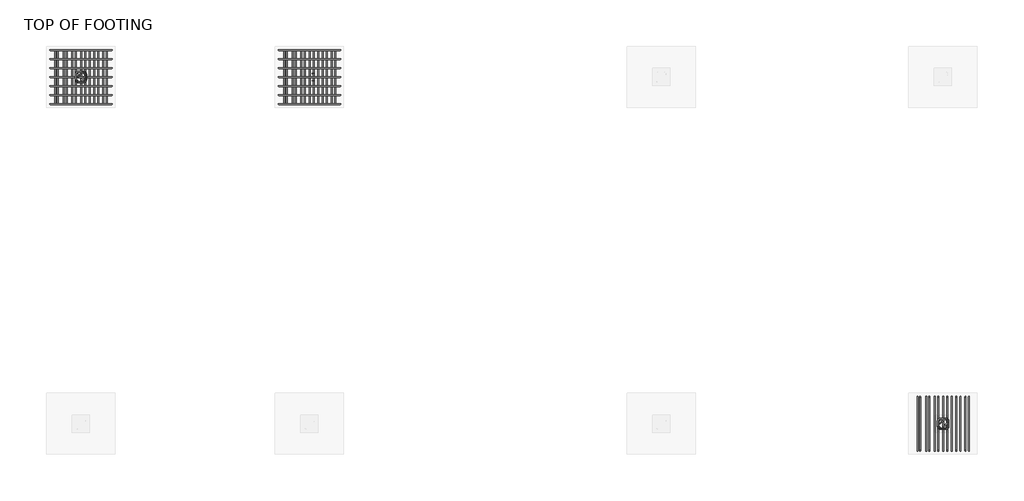
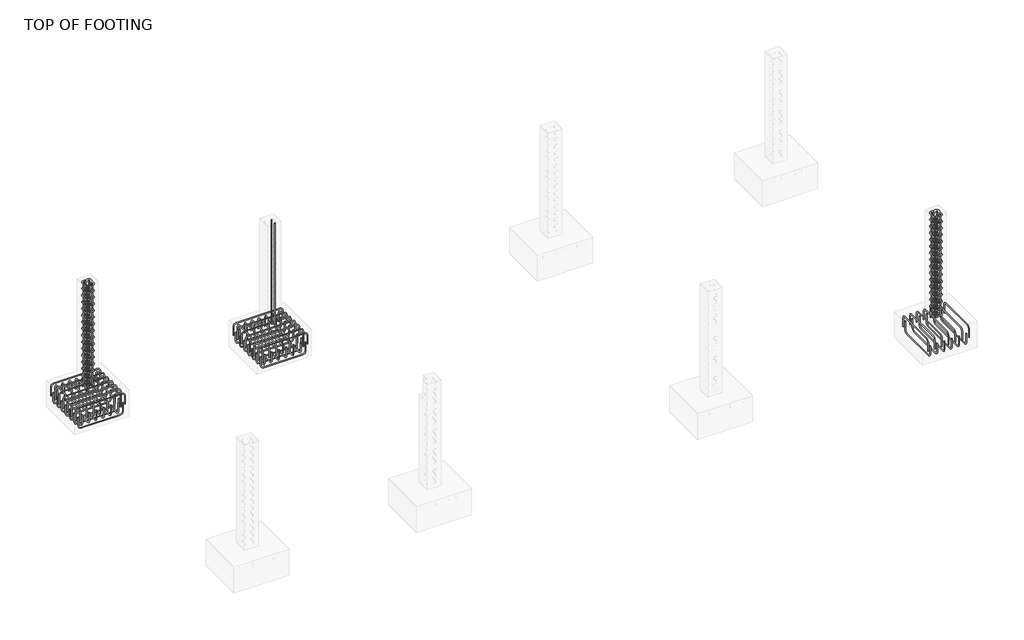
# One storey, part 5 of 6: 17 reinforcing bars.
"""IFC4 building model written with IfcOpenShell, lengths in millimetres."""

from ifc_helpers import new_model, si_unit, point, frame, origin, place, context, project, spatial, polyline, circle_curve, trimmed, segment, composite_curve, source, transform, mapped, element, save
from ifc_brep_helpers import swept_disk

model = new_model("IFC4")

# Units and contexts
model_context = context("Model", 3, world=origin())
ifc_project = project(units=[si_unit("LENGTHUNIT", "METRE", prefix="MILLI")], contexts=[model_context])

# Site, building, storey
site = spatial("IfcSite", under=ifc_project)
building = spatial("IfcBuilding", under=site)
storey = spatial("IfcBuildingStorey", under=building, Name="TOP OF FOOTING", Elevation=-1828.8)

# Reinforcing bars
placement = place(None, origin())
reinforcing_bar_shape = source(origin(), model_context, "Body", "SolidModel", [
    swept_disk(composite_curve([segment(polyline([(-14552.1855212, 4666.2516651, -2038.8), (-14552.1855212, 4666.2516651, -2186.1)]), True, "CONTINUOUS"), segment(trimmed(circle_curve(frame((-14598.5355212, 4666.2516651, -2186.1), z_axis=(0.0, 1.0, 0.0), x_axis=(46.350000000000364, 0.0, 0.0)), 46.35), [point((-14552.1855212, 4666.2516651, -2186.1))], [point((-14598.5355212, 4666.2516651, -2232.45))], True, "CARTESIAN"), True, "CONTINUOUS"), segment(polyline([(-14598.5355212, 4666.2516651, -2232.45), (-15241.6761323, 4666.2516651, -2232.45)]), True, "CONTINUOUS"), segment(trimmed(circle_curve(frame((-15241.6761323, 4666.2516651, -2186.1), z_axis=(0.0, 1.0, 0.0), x_axis=(0.0, 0.0, -46.34999999999991)), 46.35), [point((-15241.6761323, 4666.2516651, -2232.45))], [point((-15288.0261323, 4666.2516651, -2186.1))], True, "CARTESIAN"), True, "CONTINUOUS"), segment(polyline([(-15288.0261323, 4666.2516651, -2186.1), (-15288.0261323, 4666.2516651, -2038.8)]), True, "CONTINUOUS")], self_intersect=False), 6.35),
])
element("IfcReinforcingBar", 1, at=placement, inside=storey, context=model_context, shape_type="MappedRepresentation", body=[
    mapped(reinforcing_bar_shape, transform((0.0, 0.0, 0.0), x_axis=(1.0, 0.0, 0.0), y_axis=(0.0, 1.0, 0.0), z_axis=(0.0, 0.0, 1.0))),
    mapped(reinforcing_bar_shape, transform((0.0, -117.8833333, 0.0), x_axis=(1.0, 0.0, 0.0), y_axis=(0.0, 1.0, 0.0), z_axis=(0.0, 0.0, 1.0))),
    mapped(reinforcing_bar_shape, transform((0.0, -235.7666667, 0.0), x_axis=(1.0, 0.0, 0.0), y_axis=(0.0, 1.0, 0.0), z_axis=(0.0, 0.0, 1.0))),
    mapped(reinforcing_bar_shape, transform((0.0, -353.65, 0.0), x_axis=(1.0, 0.0, 0.0), y_axis=(0.0, 1.0, 0.0), z_axis=(0.0, 0.0, 1.0))),
    mapped(reinforcing_bar_shape, transform((0.0, -471.5333333, 0.0), x_axis=(1.0, 0.0, 0.0), y_axis=(0.0, 1.0, 0.0), z_axis=(0.0, 0.0, 1.0))),
    mapped(reinforcing_bar_shape, transform((0.0, -589.4166667, 0.0), x_axis=(1.0, 0.0, 0.0), y_axis=(0.0, 1.0, 0.0), z_axis=(0.0, 0.0, 1.0))),
    mapped(reinforcing_bar_shape, transform((0.0, -707.3, 0.0), x_axis=(1.0, 0.0, 0.0), y_axis=(0.0, 1.0, 0.0), z_axis=(0.0, 0.0, 1.0))),
])
reinforcing_bar_2_shape = source(origin(), model_context, "Body", "SolidModel", [
    swept_disk(composite_curve([segment(polyline([(-15327.4056799, 4666.2516651, -2070.9463075), (-15327.4056799, 4666.2516651, -1923.6463075)]), True, "CONTINUOUS"), segment(trimmed(circle_curve(frame((-15281.0556799, 4666.2516651, -1923.6463075), z_axis=(0.0, 1.0, 0.0), x_axis=(-46.350000000000364, 0.0, 0.0)), 46.35), [point((-15327.4056799, 4666.2516651, -1923.6463075))], [point((-15281.0556799, 4666.2516651, -1877.2963075))], True, "CARTESIAN"), True, "CONTINUOUS"), segment(polyline([(-15281.0556799, 4666.2516651, -1877.2963075), (-14566.4556799, 4666.2516651, -1877.2963075)]), True, "CONTINUOUS"), segment(trimmed(circle_curve(frame((-14566.4556799, 4666.2516651, -1923.6463075), z_axis=(0.0, 1.0, 0.0), x_axis=(0.0, 0.0, 46.34999999999991)), 46.35), [point((-14566.4556799, 4666.2516651, -1877.2963075))], [point((-14520.1056799, 4666.2516651, -1923.6463075))], True, "CARTESIAN"), True, "CONTINUOUS"), segment(polyline([(-14520.1056799, 4666.2516651, -1923.6463075), (-14520.1056799, 4666.2516651, -2070.9463075)]), True, "CONTINUOUS")], self_intersect=False), 6.35),
])
element("IfcReinforcingBar", 2, at=placement, inside=storey, context=model_context, shape_type="MappedRepresentation", body=[
    mapped(reinforcing_bar_2_shape, transform((0.0, 0.0, 0.0), x_axis=(1.0, 0.0, 0.0), y_axis=(0.0, 1.0, 0.0), z_axis=(0.0, 0.0, 1.0))),
    mapped(reinforcing_bar_2_shape, transform((0.0, -117.8833333, 0.0), x_axis=(1.0, 0.0, 0.0), y_axis=(0.0, 1.0, 0.0), z_axis=(0.0, 0.0, 1.0))),
    mapped(reinforcing_bar_2_shape, transform((0.0, -235.7666667, 0.0), x_axis=(1.0, 0.0, 0.0), y_axis=(0.0, 1.0, 0.0), z_axis=(0.0, 0.0, 1.0))),
    mapped(reinforcing_bar_2_shape, transform((0.0, -353.65, 0.0), x_axis=(1.0, 0.0, 0.0), y_axis=(0.0, 1.0, 0.0), z_axis=(0.0, 0.0, 1.0))),
    mapped(reinforcing_bar_2_shape, transform((0.0, -471.5333333, 0.0), x_axis=(1.0, 0.0, 0.0), y_axis=(0.0, 1.0, 0.0), z_axis=(0.0, 0.0, 1.0))),
    mapped(reinforcing_bar_2_shape, transform((0.0, -589.4166667, 0.0), x_axis=(1.0, 0.0, 0.0), y_axis=(0.0, 1.0, 0.0), z_axis=(0.0, 0.0, 1.0))),
    mapped(reinforcing_bar_2_shape, transform((0.0, -707.3, 0.0), x_axis=(1.0, 0.0, 0.0), y_axis=(0.0, 1.0, 0.0), z_axis=(0.0, 0.0, 1.0))),
])
reinforcing_bar_3_shape = source(origin(), model_context, "Body", "SolidModel", [
    swept_disk(composite_curve([segment(polyline([(-14585.2545962, 4666.2516651, -2094.0228735), (-14585.2545962, 4666.2516651, -1946.7228735)]), True, "CONTINUOUS"), segment(trimmed(circle_curve(frame((-14585.2545962, 4619.9016651, -1946.7228735), z_axis=(1.0, 0.0, 0.0), x_axis=(0.0, 46.349999999999454, 0.0)), 46.35), [point((-14585.2545962, 4666.2516651, -1946.7228735))], [point((-14585.2545962, 4619.9016651, -1900.3728735))], True, "CARTESIAN"), True, "CONTINUOUS"), segment(polyline([(-14585.2545962, 4619.9016651, -1900.3728735), (-14585.2545962, 4005.3016651, -1900.3728735)]), True, "CONTINUOUS"), segment(trimmed(circle_curve(frame((-14585.2545962, 4005.3016651, -1946.7228735), z_axis=(1.0, 0.0, 0.0), x_axis=(0.0, 0.0, 46.350000000000136)), 46.35), [point((-14585.2545962, 4005.3016651, -1900.3728735))], [point((-14585.2545962, 3958.9516651, -1946.7228735))], True, "CARTESIAN"), True, "CONTINUOUS"), segment(polyline([(-14585.2545962, 3958.9516651, -1946.7228735), (-14585.2545962, 3958.9516651, -2094.0228735)]), True, "CONTINUOUS")], self_intersect=False), 6.35),
])
element("IfcReinforcingBar", 3, at=placement, inside=storey, context=model_context, shape_type="MappedRepresentation", body=[
    mapped(reinforcing_bar_3_shape, transform((0.0, 0.0, 0.0), x_axis=(1.0, 0.0, 0.0), y_axis=(0.0, 1.0, 0.0), z_axis=(0.0, 0.0, 1.0))),
    mapped(reinforcing_bar_3_shape, transform((-112.124631, 0.0, 0.0), x_axis=(1.0, 0.0, 0.0), y_axis=(0.0, 1.0, 0.0), z_axis=(0.0, 0.0, 1.0))),
    mapped(reinforcing_bar_3_shape, transform((-224.2492621, 0.0, 0.0), x_axis=(1.0, 0.0, 0.0), y_axis=(0.0, 1.0, 0.0), z_axis=(0.0, 0.0, 1.0))),
    mapped(reinforcing_bar_3_shape, transform((-336.3738931, 0.0, 0.0), x_axis=(1.0, 0.0, 0.0), y_axis=(0.0, 1.0, 0.0), z_axis=(0.0, 0.0, 1.0))),
    mapped(reinforcing_bar_3_shape, transform((-448.4985241, 0.0, 0.0), x_axis=(1.0, 0.0, 0.0), y_axis=(0.0, 1.0, 0.0), z_axis=(0.0, 0.0, 1.0))),
    mapped(reinforcing_bar_3_shape, transform((-560.6231552, 0.0, 0.0), x_axis=(1.0, 0.0, 0.0), y_axis=(0.0, 1.0, 0.0), z_axis=(0.0, 0.0, 1.0))),
    mapped(reinforcing_bar_3_shape, transform((-672.7477862, 0.0, 0.0), x_axis=(1.0, 0.0, 0.0), y_axis=(0.0, 1.0, 0.0), z_axis=(0.0, 0.0, 1.0))),
])
reinforcing_bar_4_shape = source(origin(), model_context, "Body", "SolidModel", [
    swept_disk(composite_curve([segment(polyline([(-15225.2448384, 4666.2516651, -2014.7438142), (-15225.2448384, 4666.2516651, -2162.0438142)]), True, "CONTINUOUS"), segment(trimmed(circle_curve(frame((-15225.2448384, 4619.9016651, -2162.0438142), z_axis=(-1.0, 0.0, 0.0), x_axis=(0.0, 46.349999999999454, 0.0)), 46.35), [point((-15225.2448384, 4666.2516651, -2162.0438142))], [point((-15225.2448384, 4619.9016651, -2208.3938142))], True, "CARTESIAN"), True, "CONTINUOUS"), segment(polyline([(-15225.2448384, 4619.9016651, -2208.3938142), (-15225.2448384, 4005.3016651, -2208.3938142)]), True, "CONTINUOUS"), segment(trimmed(circle_curve(frame((-15225.2448384, 4005.3016651, -2162.0438142), z_axis=(-1.0, 0.0, 0.0), x_axis=(0.0, 0.0, -46.350000000000364)), 46.35), [point((-15225.2448384, 4005.3016651, -2208.3938142))], [point((-15225.2448384, 3958.9516651, -2162.0438142))], True, "CARTESIAN"), True, "CONTINUOUS"), segment(polyline([(-15225.2448384, 3958.9516651, -2162.0438142), (-15225.2448384, 3958.9516651, -2014.7438142)]), True, "CONTINUOUS")], self_intersect=False), 6.35),
])
element("IfcReinforcingBar", 4, at=placement, inside=storey, context=model_context, shape_type="MappedRepresentation", body=[
    mapped(reinforcing_bar_4_shape, transform((0.0, 0.0, 0.0), x_axis=(1.0, 0.0, 0.0), y_axis=(0.0, 1.0, 0.0), z_axis=(0.0, 0.0, 1.0))),
    mapped(reinforcing_bar_4_shape, transform((118.647936, 0.0, 0.0), x_axis=(1.0, 0.0, 0.0), y_axis=(0.0, 1.0, 0.0), z_axis=(0.0, 0.0, 1.0))),
    mapped(reinforcing_bar_4_shape, transform((237.295872, 0.0, 0.0), x_axis=(1.0, 0.0, 0.0), y_axis=(0.0, 1.0, 0.0), z_axis=(0.0, 0.0, 1.0))),
    mapped(reinforcing_bar_4_shape, transform((355.943808, 0.0, 0.0), x_axis=(1.0, 0.0, 0.0), y_axis=(0.0, 1.0, 0.0), z_axis=(0.0, 0.0, 1.0))),
    mapped(reinforcing_bar_4_shape, transform((474.591744, 0.0, 0.0), x_axis=(1.0, 0.0, 0.0), y_axis=(0.0, 1.0, 0.0), z_axis=(0.0, 0.0, 1.0))),
    mapped(reinforcing_bar_4_shape, transform((593.23968, 0.0, 0.0), x_axis=(1.0, 0.0, 0.0), y_axis=(0.0, 1.0, 0.0), z_axis=(0.0, 0.0, 1.0))),
])
reinforcing_bar_5_shape = source(origin(), model_context, "Body", "SolidModel", [
    swept_disk(composite_curve([segment(polyline([(-11554.9855212, 4666.2516651, -2038.8), (-11554.9855212, 4666.2516651, -2186.1)]), True, "CONTINUOUS"), segment(trimmed(circle_curve(frame((-11601.3355212, 4666.2516651, -2186.1), z_axis=(0.0, 1.0, 0.0), x_axis=(46.350000000000364, 0.0, 0.0)), 46.35), [point((-11554.9855212, 4666.2516651, -2186.1))], [point((-11601.3355212, 4666.2516651, -2232.45))], True, "CARTESIAN"), True, "CONTINUOUS"), segment(polyline([(-11601.3355212, 4666.2516651, -2232.45), (-12244.4761323, 4666.2516651, -2232.45)]), True, "CONTINUOUS"), segment(trimmed(circle_curve(frame((-12244.4761323, 4666.2516651, -2186.1), z_axis=(0.0, 1.0, 0.0), x_axis=(0.0, 0.0, -46.34999999999991)), 46.35), [point((-12244.4761323, 4666.2516651, -2232.45))], [point((-12290.8261323, 4666.2516651, -2186.1))], True, "CARTESIAN"), True, "CONTINUOUS"), segment(polyline([(-12290.8261323, 4666.2516651, -2186.1), (-12290.8261323, 4666.2516651, -2038.8)]), True, "CONTINUOUS")], self_intersect=False), 6.35),
])
element("IfcReinforcingBar", 5, at=placement, inside=storey, context=model_context, shape_type="MappedRepresentation", body=[
    mapped(reinforcing_bar_5_shape, transform((0.0, 0.0, 0.0), x_axis=(1.0, 0.0, 0.0), y_axis=(0.0, 1.0, 0.0), z_axis=(0.0, 0.0, 1.0))),
    mapped(reinforcing_bar_5_shape, transform((0.0, -117.8833333, 0.0), x_axis=(1.0, 0.0, 0.0), y_axis=(0.0, 1.0, 0.0), z_axis=(0.0, 0.0, 1.0))),
    mapped(reinforcing_bar_5_shape, transform((0.0, -235.7666667, 0.0), x_axis=(1.0, 0.0, 0.0), y_axis=(0.0, 1.0, 0.0), z_axis=(0.0, 0.0, 1.0))),
    mapped(reinforcing_bar_5_shape, transform((0.0, -353.65, 0.0), x_axis=(1.0, 0.0, 0.0), y_axis=(0.0, 1.0, 0.0), z_axis=(0.0, 0.0, 1.0))),
    mapped(reinforcing_bar_5_shape, transform((0.0, -471.5333333, 0.0), x_axis=(1.0, 0.0, 0.0), y_axis=(0.0, 1.0, 0.0), z_axis=(0.0, 0.0, 1.0))),
    mapped(reinforcing_bar_5_shape, transform((0.0, -589.4166667, 0.0), x_axis=(1.0, 0.0, 0.0), y_axis=(0.0, 1.0, 0.0), z_axis=(0.0, 0.0, 1.0))),
    mapped(reinforcing_bar_5_shape, transform((0.0, -707.3, 0.0), x_axis=(1.0, 0.0, 0.0), y_axis=(0.0, 1.0, 0.0), z_axis=(0.0, 0.0, 1.0))),
])
reinforcing_bar_6_shape = source(origin(), model_context, "Body", "SolidModel", [
    swept_disk(composite_curve([segment(polyline([(-12330.2056799, 4666.2516651, -2070.9463075), (-12330.2056799, 4666.2516651, -1923.6463075)]), True, "CONTINUOUS"), segment(trimmed(circle_curve(frame((-12283.8556799, 4666.2516651, -1923.6463075), z_axis=(0.0, 1.0, 0.0), x_axis=(-46.350000000000364, 0.0, 0.0)), 46.35), [point((-12330.2056799, 4666.2516651, -1923.6463075))], [point((-12283.8556799, 4666.2516651, -1877.2963075))], True, "CARTESIAN"), True, "CONTINUOUS"), segment(polyline([(-12283.8556799, 4666.2516651, -1877.2963075), (-11569.2556799, 4666.2516651, -1877.2963075)]), True, "CONTINUOUS"), segment(trimmed(circle_curve(frame((-11569.2556799, 4666.2516651, -1923.6463075), z_axis=(0.0, 1.0, 0.0), x_axis=(0.0, 0.0, 46.34999999999991)), 46.35), [point((-11569.2556799, 4666.2516651, -1877.2963075))], [point((-11522.9056799, 4666.2516651, -1923.6463075))], True, "CARTESIAN"), True, "CONTINUOUS"), segment(polyline([(-11522.9056799, 4666.2516651, -1923.6463075), (-11522.9056799, 4666.2516651, -2070.9463075)]), True, "CONTINUOUS")], self_intersect=False), 6.35),
])
element("IfcReinforcingBar", 6, at=placement, inside=storey, context=model_context, shape_type="MappedRepresentation", body=[
    mapped(reinforcing_bar_6_shape, transform((0.0, 0.0, 0.0), x_axis=(1.0, 0.0, 0.0), y_axis=(0.0, 1.0, 0.0), z_axis=(0.0, 0.0, 1.0))),
    mapped(reinforcing_bar_6_shape, transform((0.0, -117.8833333, 0.0), x_axis=(1.0, 0.0, 0.0), y_axis=(0.0, 1.0, 0.0), z_axis=(0.0, 0.0, 1.0))),
    mapped(reinforcing_bar_6_shape, transform((0.0, -235.7666667, 0.0), x_axis=(1.0, 0.0, 0.0), y_axis=(0.0, 1.0, 0.0), z_axis=(0.0, 0.0, 1.0))),
    mapped(reinforcing_bar_6_shape, transform((0.0, -353.65, 0.0), x_axis=(1.0, 0.0, 0.0), y_axis=(0.0, 1.0, 0.0), z_axis=(0.0, 0.0, 1.0))),
    mapped(reinforcing_bar_6_shape, transform((0.0, -471.5333333, 0.0), x_axis=(1.0, 0.0, 0.0), y_axis=(0.0, 1.0, 0.0), z_axis=(0.0, 0.0, 1.0))),
    mapped(reinforcing_bar_6_shape, transform((0.0, -589.4166667, 0.0), x_axis=(1.0, 0.0, 0.0), y_axis=(0.0, 1.0, 0.0), z_axis=(0.0, 0.0, 1.0))),
    mapped(reinforcing_bar_6_shape, transform((0.0, -707.3, 0.0), x_axis=(1.0, 0.0, 0.0), y_axis=(0.0, 1.0, 0.0), z_axis=(0.0, 0.0, 1.0))),
])
reinforcing_bar_7_shape = source(origin(), model_context, "Body", "SolidModel", [
    swept_disk(composite_curve([segment(polyline([(-11588.0545962, 4666.2516651, -2094.0228735), (-11588.0545962, 4666.2516651, -1946.7228735)]), True, "CONTINUOUS"), segment(trimmed(circle_curve(frame((-11588.0545962, 4619.9016651, -1946.7228735), z_axis=(1.0, 0.0, 0.0), x_axis=(0.0, 46.349999999999454, 0.0)), 46.35), [point((-11588.0545962, 4666.2516651, -1946.7228735))], [point((-11588.0545962, 4619.9016651, -1900.3728735))], True, "CARTESIAN"), True, "CONTINUOUS"), segment(polyline([(-11588.0545962, 4619.9016651, -1900.3728735), (-11588.0545962, 4005.3016651, -1900.3728735)]), True, "CONTINUOUS"), segment(trimmed(circle_curve(frame((-11588.0545962, 4005.3016651, -1946.7228735), z_axis=(1.0, 0.0, 0.0), x_axis=(0.0, 0.0, 46.350000000000136)), 46.35), [point((-11588.0545962, 4005.3016651, -1900.3728735))], [point((-11588.0545962, 3958.9516651, -1946.7228735))], True, "CARTESIAN"), True, "CONTINUOUS"), segment(polyline([(-11588.0545962, 3958.9516651, -1946.7228735), (-11588.0545962, 3958.9516651, -2094.0228735)]), True, "CONTINUOUS")], self_intersect=False), 6.35),
])
element("IfcReinforcingBar", 7, at=placement, inside=storey, context=model_context, shape_type="MappedRepresentation", body=[
    mapped(reinforcing_bar_7_shape, transform((0.0, 0.0, 0.0), x_axis=(1.0, 0.0, 0.0), y_axis=(0.0, 1.0, 0.0), z_axis=(0.0, 0.0, 1.0))),
    mapped(reinforcing_bar_7_shape, transform((-112.124631, 0.0, 0.0), x_axis=(1.0, 0.0, 0.0), y_axis=(0.0, 1.0, 0.0), z_axis=(0.0, 0.0, 1.0))),
    mapped(reinforcing_bar_7_shape, transform((-224.2492621, 0.0, 0.0), x_axis=(1.0, 0.0, 0.0), y_axis=(0.0, 1.0, 0.0), z_axis=(0.0, 0.0, 1.0))),
    mapped(reinforcing_bar_7_shape, transform((-336.3738931, 0.0, 0.0), x_axis=(1.0, 0.0, 0.0), y_axis=(0.0, 1.0, 0.0), z_axis=(0.0, 0.0, 1.0))),
    mapped(reinforcing_bar_7_shape, transform((-448.4985241, 0.0, 0.0), x_axis=(1.0, 0.0, 0.0), y_axis=(0.0, 1.0, 0.0), z_axis=(0.0, 0.0, 1.0))),
    mapped(reinforcing_bar_7_shape, transform((-560.6231552, 0.0, 0.0), x_axis=(1.0, 0.0, 0.0), y_axis=(0.0, 1.0, 0.0), z_axis=(0.0, 0.0, 1.0))),
    mapped(reinforcing_bar_7_shape, transform((-672.7477862, 0.0, 0.0), x_axis=(1.0, 0.0, 0.0), y_axis=(0.0, 1.0, 0.0), z_axis=(0.0, 0.0, 1.0))),
])
reinforcing_bar_8_shape = source(origin(), model_context, "Body", "SolidModel", [
    swept_disk(composite_curve([segment(polyline([(-12228.0448384, 4666.2516651, -2014.7438142), (-12228.0448384, 4666.2516651, -2162.0438142)]), True, "CONTINUOUS"), segment(trimmed(circle_curve(frame((-12228.0448384, 4619.9016651, -2162.0438142), z_axis=(-1.0, 0.0, 0.0), x_axis=(0.0, 46.349999999999454, 0.0)), 46.35), [point((-12228.0448384, 4666.2516651, -2162.0438142))], [point((-12228.0448384, 4619.9016651, -2208.3938142))], True, "CARTESIAN"), True, "CONTINUOUS"), segment(polyline([(-12228.0448384, 4619.9016651, -2208.3938142), (-12228.0448384, 4005.3016651, -2208.3938142)]), True, "CONTINUOUS"), segment(trimmed(circle_curve(frame((-12228.0448384, 4005.3016651, -2162.0438142), z_axis=(-1.0, 0.0, 0.0), x_axis=(0.0, 0.0, -46.350000000000364)), 46.35), [point((-12228.0448384, 4005.3016651, -2208.3938142))], [point((-12228.0448384, 3958.9516651, -2162.0438142))], True, "CARTESIAN"), True, "CONTINUOUS"), segment(polyline([(-12228.0448384, 3958.9516651, -2162.0438142), (-12228.0448384, 3958.9516651, -2014.7438142)]), True, "CONTINUOUS")], self_intersect=False), 6.35),
])
element("IfcReinforcingBar", 8, at=placement, inside=storey, context=model_context, shape_type="MappedRepresentation", body=[
    mapped(reinforcing_bar_8_shape, transform((0.0, 0.0, 0.0), x_axis=(1.0, 0.0, 0.0), y_axis=(0.0, 1.0, 0.0), z_axis=(0.0, 0.0, 1.0))),
    mapped(reinforcing_bar_8_shape, transform((118.647936, 0.0, 0.0), x_axis=(1.0, 0.0, 0.0), y_axis=(0.0, 1.0, 0.0), z_axis=(0.0, 0.0, 1.0))),
    mapped(reinforcing_bar_8_shape, transform((237.295872, 0.0, 0.0), x_axis=(1.0, 0.0, 0.0), y_axis=(0.0, 1.0, 0.0), z_axis=(0.0, 0.0, 1.0))),
    mapped(reinforcing_bar_8_shape, transform((355.943808, 0.0, 0.0), x_axis=(1.0, 0.0, 0.0), y_axis=(0.0, 1.0, 0.0), z_axis=(0.0, 0.0, 1.0))),
    mapped(reinforcing_bar_8_shape, transform((474.591744, 0.0, 0.0), x_axis=(1.0, 0.0, 0.0), y_axis=(0.0, 1.0, 0.0), z_axis=(0.0, 0.0, 1.0))),
    mapped(reinforcing_bar_8_shape, transform((593.23968, 0.0, 0.0), x_axis=(1.0, 0.0, 0.0), y_axis=(0.0, 1.0, 0.0), z_axis=(0.0, 0.0, 1.0))),
])
reinforcing_bar_9_shape = source(origin(), model_context, "Body", "SolidModel", [
    swept_disk(composite_curve([segment(polyline([(-3282.2545962, 120.9474721, -2094.0228735), (-3282.2545962, 120.9474721, -1946.7228735)]), True, "CONTINUOUS"), segment(trimmed(circle_curve(frame((-3282.2545962, 74.5974721, -1946.7228735), z_axis=(1.0, 0.0, 0.0), x_axis=(0.0, 46.349999999999994, 0.0)), 46.35), [point((-3282.2545962, 120.9474721, -1946.7228735))], [point((-3282.2545962, 74.5974721, -1900.3728735))], True, "CARTESIAN"), True, "CONTINUOUS"), segment(polyline([(-3282.2545962, 74.5974721, -1900.3728735), (-3282.2545962, -540.0025279, -1900.3728735)]), True, "CONTINUOUS"), segment(trimmed(circle_curve(frame((-3282.2545962, -540.0025279, -1946.7228735), z_axis=(1.0, 0.0, 0.0), x_axis=(0.0, 0.0, 46.350000000000136)), 46.35), [point((-3282.2545962, -540.0025279, -1900.3728735))], [point((-3282.2545962, -586.3525279, -1946.7228735))], True, "CARTESIAN"), True, "CONTINUOUS"), segment(polyline([(-3282.2545962, -586.3525279, -1946.7228735), (-3282.2545962, -586.3525279, -2094.0228735)]), True, "CONTINUOUS")], self_intersect=False), 6.35),
])
element("IfcReinforcingBar", 9, at=placement, inside=storey, context=model_context, shape_type="MappedRepresentation", body=[
    mapped(reinforcing_bar_9_shape, transform((0.0, 0.0, 0.0), x_axis=(1.0, 0.0, 0.0), y_axis=(0.0, 1.0, 0.0), z_axis=(0.0, 0.0, 1.0))),
    mapped(reinforcing_bar_9_shape, transform((-112.124631, 0.0, 0.0), x_axis=(1.0, 0.0, 0.0), y_axis=(0.0, 1.0, 0.0), z_axis=(0.0, 0.0, 1.0))),
    mapped(reinforcing_bar_9_shape, transform((-224.2492621, 0.0, 0.0), x_axis=(1.0, 0.0, 0.0), y_axis=(0.0, 1.0, 0.0), z_axis=(0.0, 0.0, 1.0))),
    mapped(reinforcing_bar_9_shape, transform((-336.3738931, 0.0, 0.0), x_axis=(1.0, 0.0, 0.0), y_axis=(0.0, 1.0, 0.0), z_axis=(0.0, 0.0, 1.0))),
    mapped(reinforcing_bar_9_shape, transform((-448.4985241, 0.0, 0.0), x_axis=(1.0, 0.0, 0.0), y_axis=(0.0, 1.0, 0.0), z_axis=(0.0, 0.0, 1.0))),
    mapped(reinforcing_bar_9_shape, transform((-560.6231552, 0.0, 0.0), x_axis=(1.0, 0.0, 0.0), y_axis=(0.0, 1.0, 0.0), z_axis=(0.0, 0.0, 1.0))),
    mapped(reinforcing_bar_9_shape, transform((-672.7477862, 0.0, 0.0), x_axis=(1.0, 0.0, 0.0), y_axis=(0.0, 1.0, 0.0), z_axis=(0.0, 0.0, 1.0))),
])
reinforcing_bar_10_shape = source(origin(), model_context, "Body", "SolidModel", [
    swept_disk(composite_curve([segment(polyline([(-3922.2448384, 120.9474721, -2014.7438142), (-3922.2448384, 120.9474721, -2162.0438142)]), True, "CONTINUOUS"), segment(trimmed(circle_curve(frame((-3922.2448384, 74.5974721, -2162.0438142), z_axis=(-1.0, 0.0, 0.0), x_axis=(0.0, 46.349999999999994, 0.0)), 46.35), [point((-3922.2448384, 120.9474721, -2162.0438142))], [point((-3922.2448384, 74.5974721, -2208.3938142))], True, "CARTESIAN"), True, "CONTINUOUS"), segment(polyline([(-3922.2448384, 74.5974721, -2208.3938142), (-3922.2448384, -540.0025279, -2208.3938142)]), True, "CONTINUOUS"), segment(trimmed(circle_curve(frame((-3922.2448384, -540.0025279, -2162.0438142), z_axis=(-1.0, 0.0, 0.0), x_axis=(0.0, 0.0, -46.350000000000364)), 46.35), [point((-3922.2448384, -540.0025279, -2208.3938142))], [point((-3922.2448384, -586.3525279, -2162.0438142))], True, "CARTESIAN"), True, "CONTINUOUS"), segment(polyline([(-3922.2448384, -586.3525279, -2162.0438142), (-3922.2448384, -586.3525279, -2014.7438142)]), True, "CONTINUOUS")], self_intersect=False), 6.35),
])
element("IfcReinforcingBar", 10, at=placement, inside=storey, context=model_context, shape_type="MappedRepresentation", body=[
    mapped(reinforcing_bar_10_shape, transform((0.0, 0.0, 0.0), x_axis=(1.0, 0.0, 0.0), y_axis=(0.0, 1.0, 0.0), z_axis=(0.0, 0.0, 1.0))),
    mapped(reinforcing_bar_10_shape, transform((118.647936, 0.0, 0.0), x_axis=(1.0, 0.0, 0.0), y_axis=(0.0, 1.0, 0.0), z_axis=(0.0, 0.0, 1.0))),
    mapped(reinforcing_bar_10_shape, transform((237.295872, 0.0, 0.0), x_axis=(1.0, 0.0, 0.0), y_axis=(0.0, 1.0, 0.0), z_axis=(0.0, 0.0, 1.0))),
    mapped(reinforcing_bar_10_shape, transform((355.943808, 0.0, 0.0), x_axis=(1.0, 0.0, 0.0), y_axis=(0.0, 1.0, 0.0), z_axis=(0.0, 0.0, 1.0))),
    mapped(reinforcing_bar_10_shape, transform((474.591744, 0.0, 0.0), x_axis=(1.0, 0.0, 0.0), y_axis=(0.0, 1.0, 0.0), z_axis=(0.0, 0.0, 1.0))),
    mapped(reinforcing_bar_10_shape, transform((593.23968, 0.0, 0.0), x_axis=(1.0, 0.0, 0.0), y_axis=(0.0, 1.0, 0.0), z_axis=(0.0, 0.0, 1.0))),
])
reinforcing_bar_11_shape = source(origin(), model_context, "Body", "SolidModel", [
    swept_disk(composite_curve([segment(polyline([(-11881.8006936, 4361.3993608, -40.0), (-11881.8006936, 4361.3993608, -1788.8)]), True, "CONTINUOUS")], self_intersect=False), 6.35),
])
element("IfcReinforcingBar", 11, at=placement, inside=storey, context=model_context, shape_type="MappedRepresentation", body=[
    mapped(reinforcing_bar_11_shape, transform((0.0, 0.0, 0.0), x_axis=(1.0, 0.0, 0.0), y_axis=(0.0, 1.0, 0.0), z_axis=(0.0, 0.0, 1.0))),
    mapped(reinforcing_bar_11_shape, transform((0.0, -96.9916148, 0.0), x_axis=(1.0, 0.0, 0.0), y_axis=(0.0, 1.0, 0.0), z_axis=(0.0, 0.0, 1.0))),
])
reinforcing_bar_12_shape = source(origin(), model_context, "Body", "SolidModel", [
    swept_disk(composite_curve([segment(polyline([(-14879.0006936, 4361.3993608, -40.0), (-14879.0006936, 4361.3993608, -1788.8)]), True, "CONTINUOUS")], self_intersect=False), 6.35),
])
element("IfcReinforcingBar", 12, at=placement, inside=storey, context=model_context, shape_type="MappedRepresentation", body=[
    mapped(reinforcing_bar_12_shape, transform((0.0, 0.0, 0.0), x_axis=(1.0, 0.0, 0.0), y_axis=(0.0, 1.0, 0.0), z_axis=(0.0, 0.0, 1.0))),
    mapped(reinforcing_bar_12_shape, transform((0.0, -96.9916148, 0.0), x_axis=(1.0, 0.0, 0.0), y_axis=(0.0, 1.0, 0.0), z_axis=(0.0, 0.0, 1.0))),
])
reinforcing_bar_13_shape = source(origin(), model_context, "Body", "SolidModel", [
    swept_disk(composite_curve([segment(polyline([(-14965.0670404, 4315.6258997, -46.35), (-14909.3234775, 4371.3694627, -46.35)]), True, "CONTINUOUS"), segment(trimmed(circle_curve(frame((-14887.1556799, 4349.2016651, -46.35), z_axis=(0.0, 0.0, -1.0), x_axis=(-22.167797599999176, 22.167797600000085, 0.0)), 31.35), [point((-14909.3234775, 4371.3694627, -46.35))], [point((-14855.8056799, 4349.2016651, -46.35))], True, "CARTESIAN"), True, "CONTINUOUS"), segment(polyline([(-14855.8056799, 4349.2016651, -46.35), (-14855.8056799, 4276.0016651, -46.35)]), True, "CONTINUOUS"), segment(trimmed(circle_curve(frame((-14887.1556799, 4276.0016651, -46.35), z_axis=(0.0, 0.0, -1.0), x_axis=(31.350000000000364, 0.0, 0.0)), 31.35), [point((-14855.8056799, 4276.0016651, -46.35))], [point((-14887.1556799, 4244.6516651, -46.35))], True, "CARTESIAN"), True, "CONTINUOUS"), segment(polyline([(-14887.1556799, 4244.6516651, -46.35), (-14960.3556799, 4244.6516651, -46.35)]), True, "CONTINUOUS"), segment(trimmed(circle_curve(frame((-14960.3556799, 4275.8656639, -43.4330185), z_axis=(0.0, 0.09304566152621355, -0.9956618426308951), x_axis=(0.0, -31.2139987999999, -2.9169814999999986)), 31.35), [point((-14960.3556799, 4244.6516651, -46.35))], [point((-14991.7056799, 4275.8656639, -43.4330185))], True, "CARTESIAN"), True, "CONTINUOUS"), segment(polyline([(-14991.7056799, 4275.8656639, -43.4330185), (-14991.7056799, 4349.3376663, -36.5669815)]), True, "CONTINUOUS"), segment(trimmed(circle_curve(frame((-14960.3556799, 4349.3376663, -36.5669815), z_axis=(0.0, 0.09304566152621355, -0.9956618426308951), x_axis=(-31.350000000000364, 0.0, 0.0)), 31.35), [point((-14991.7056799, 4349.3376663, -36.5669815))], [point((-14960.3556799, 4380.5516651, -33.65))], True, "CARTESIAN"), True, "CONTINUOUS"), segment(polyline([(-14960.3556799, 4380.5516651, -33.65), (-14887.1556799, 4380.5516651, -33.65)]), True, "CONTINUOUS"), segment(trimmed(circle_curve(frame((-14887.1556799, 4349.2016651, -33.65), z_axis=(0.0, 0.0, -1.0), x_axis=(0.0, 31.349999999999454, 0.0)), 31.35), [point((-14887.1556799, 4380.5516651, -33.65))], [point((-14864.9878823, 4327.0338675, -33.65))], True, "CARTESIAN"), True, "CONTINUOUS"), segment(polyline([(-14864.9878823, 4327.0338675, -33.65), (-14920.7314452, 4271.2903046, -33.65)]), True, "CONTINUOUS")], self_intersect=False), 6.35),
])
element("IfcReinforcingBar", 13, at=placement, inside=storey, context=model_context, shape_type="MappedRepresentation", body=[
    mapped(reinforcing_bar_13_shape, transform((0.0, 0.0, 0.0), x_axis=(1.0, 0.0, 0.0), y_axis=(0.0, 1.0, 0.0), z_axis=(0.0, 0.0, 1.0))),
    mapped(reinforcing_bar_13_shape, transform((0.0, 0.0, -115.74), x_axis=(1.0, 0.0, 0.0), y_axis=(0.0, 1.0, 0.0), z_axis=(0.0, 0.0, 1.0))),
    mapped(reinforcing_bar_13_shape, transform((0.0, 0.0, -231.48), x_axis=(1.0, 0.0, 0.0), y_axis=(0.0, 1.0, 0.0), z_axis=(0.0, 0.0, 1.0))),
    mapped(reinforcing_bar_13_shape, transform((0.0, 0.0, -347.22), x_axis=(1.0, 0.0, 0.0), y_axis=(0.0, 1.0, 0.0), z_axis=(0.0, 0.0, 1.0))),
    mapped(reinforcing_bar_13_shape, transform((0.0, 0.0, -462.96), x_axis=(1.0, 0.0, 0.0), y_axis=(0.0, 1.0, 0.0), z_axis=(0.0, 0.0, 1.0))),
    mapped(reinforcing_bar_13_shape, transform((0.0, 0.0, -578.7), x_axis=(1.0, 0.0, 0.0), y_axis=(0.0, 1.0, 0.0), z_axis=(0.0, 0.0, 1.0))),
    mapped(reinforcing_bar_13_shape, transform((0.0, 0.0, -694.44), x_axis=(1.0, 0.0, 0.0), y_axis=(0.0, 1.0, 0.0), z_axis=(0.0, 0.0, 1.0))),
    mapped(reinforcing_bar_13_shape, transform((0.0, 0.0, -810.18), x_axis=(1.0, 0.0, 0.0), y_axis=(0.0, 1.0, 0.0), z_axis=(0.0, 0.0, 1.0))),
    mapped(reinforcing_bar_13_shape, transform((0.0, 0.0, -925.92), x_axis=(1.0, 0.0, 0.0), y_axis=(0.0, 1.0, 0.0), z_axis=(0.0, 0.0, 1.0))),
    mapped(reinforcing_bar_13_shape, transform((0.0, 0.0, -1041.66), x_axis=(1.0, 0.0, 0.0), y_axis=(0.0, 1.0, 0.0), z_axis=(0.0, 0.0, 1.0))),
    mapped(reinforcing_bar_13_shape, transform((0.0, 0.0, -1157.4), x_axis=(1.0, 0.0, 0.0), y_axis=(0.0, 1.0, 0.0), z_axis=(0.0, 0.0, 1.0))),
    mapped(reinforcing_bar_13_shape, transform((0.0, 0.0, -1273.14), x_axis=(1.0, 0.0, 0.0), y_axis=(0.0, 1.0, 0.0), z_axis=(0.0, 0.0, 1.0))),
    mapped(reinforcing_bar_13_shape, transform((0.0, 0.0, -1388.88), x_axis=(1.0, 0.0, 0.0), y_axis=(0.0, 1.0, 0.0), z_axis=(0.0, 0.0, 1.0))),
    mapped(reinforcing_bar_13_shape, transform((0.0, 0.0, -1504.62), x_axis=(1.0, 0.0, 0.0), y_axis=(0.0, 1.0, 0.0), z_axis=(0.0, 0.0, 1.0))),
    mapped(reinforcing_bar_13_shape, transform((0.0, 0.0, -1620.36), x_axis=(1.0, 0.0, 0.0), y_axis=(0.0, 1.0, 0.0), z_axis=(0.0, 0.0, 1.0))),
    mapped(reinforcing_bar_13_shape, transform((0.0, 0.0, -1736.1), x_axis=(1.0, 0.0, 0.0), y_axis=(0.0, 1.0, 0.0), z_axis=(0.0, 0.0, 1.0))),
])
reinforcing_bar_14_shape = source(origin(), model_context, "Body", "SolidModel", [
    swept_disk(composite_curve([segment(polyline([(-14968.5106662, 4361.3993608, -40.0), (-14968.5106662, 4361.3993608, -1788.8)]), True, "CONTINUOUS")], self_intersect=False), 6.35),
])
element("IfcReinforcingBar", 14, at=placement, inside=storey, context=model_context, shape_type="MappedRepresentation", body=[
    mapped(reinforcing_bar_14_shape, transform((0.0, 0.0, 0.0), x_axis=(1.0, 0.0, 0.0), y_axis=(0.0, 1.0, 0.0), z_axis=(0.0, 0.0, 1.0))),
    mapped(reinforcing_bar_14_shape, transform((0.0, -96.9916148, 0.0), x_axis=(1.0, 0.0, 0.0), y_axis=(0.0, 1.0, 0.0), z_axis=(0.0, 0.0, 1.0))),
])
reinforcing_bar_15_shape = source(origin(), model_context, "Body", "SolidModel", [
    swept_disk(composite_curve([segment(polyline([(-3576.0006936, -183.9048321, -40.0), (-3576.0006936, -183.9048321, -1788.8)]), True, "CONTINUOUS")], self_intersect=False), 6.35),
])
element("IfcReinforcingBar", 15, at=placement, inside=storey, context=model_context, shape_type="MappedRepresentation", body=[
    mapped(reinforcing_bar_15_shape, transform((0.0, 0.0, 0.0), x_axis=(1.0, 0.0, 0.0), y_axis=(0.0, 1.0, 0.0), z_axis=(0.0, 0.0, 1.0))),
    mapped(reinforcing_bar_15_shape, transform((0.0, -96.9916148, 0.0), x_axis=(1.0, 0.0, 0.0), y_axis=(0.0, 1.0, 0.0), z_axis=(0.0, 0.0, 1.0))),
])
reinforcing_bar_16_shape = source(origin(), model_context, "Body", "SolidModel", [
    swept_disk(composite_curve([segment(polyline([(-3662.0670404, -229.6782932, -46.35), (-3606.3234775, -173.9347303, -46.35)]), True, "CONTINUOUS"), segment(trimmed(circle_curve(frame((-3584.1556799, -196.1025279, -46.35), z_axis=(0.0, 0.0, -1.0), x_axis=(-22.167797600000085, 22.1677976, 0.0)), 31.35), [point((-3606.3234775, -173.9347303, -46.35))], [point((-3552.8056799, -196.1025279, -46.35))], True, "CARTESIAN"), True, "CONTINUOUS"), segment(polyline([(-3552.8056799, -196.1025279, -46.35), (-3552.8056799, -269.3025279, -46.35)]), True, "CONTINUOUS"), segment(trimmed(circle_curve(frame((-3584.1556799, -269.3025279, -46.35), z_axis=(0.0, 0.0, -1.0), x_axis=(31.34999999999991, 0.0, 0.0)), 31.35), [point((-3552.8056799, -269.3025279, -46.35))], [point((-3584.1556799, -300.6525279, -46.35))], True, "CARTESIAN"), True, "CONTINUOUS"), segment(polyline([(-3584.1556799, -300.6525279, -46.35), (-3657.3556799, -300.6525279, -46.35)]), True, "CONTINUOUS"), segment(trimmed(circle_curve(frame((-3657.3556799, -269.4385291, -43.4330185), z_axis=(0.0, 0.09304566152621355, -0.9956618426308951), x_axis=(0.0, -31.213998800000013, -2.9169814999999986)), 31.35), [point((-3657.3556799, -300.6525279, -46.35))], [point((-3688.7056799, -269.4385291, -43.4330185))], True, "CARTESIAN"), True, "CONTINUOUS"), segment(polyline([(-3688.7056799, -269.4385291, -43.4330185), (-3688.7056799, -195.9665266, -36.5669815)]), True, "CONTINUOUS"), segment(trimmed(circle_curve(frame((-3657.3556799, -195.9665266, -36.5669815), z_axis=(0.0, 0.09304566152621355, -0.9956618426308951), x_axis=(-31.350000000000364, 0.0, 0.0)), 31.35), [point((-3688.7056799, -195.9665266, -36.5669815))], [point((-3657.3556799, -164.7525279, -33.65))], True, "CARTESIAN"), True, "CONTINUOUS"), segment(polyline([(-3657.3556799, -164.7525279, -33.65), (-3584.1556799, -164.7525279, -33.65)]), True, "CONTINUOUS"), segment(trimmed(circle_curve(frame((-3584.1556799, -196.1025279, -33.65), z_axis=(0.0, 0.0, -1.0), x_axis=(0.0, 31.350000000000023, 0.0)), 31.35), [point((-3584.1556799, -164.7525279, -33.65))], [point((-3561.9878823, -218.2703255, -33.65))], True, "CARTESIAN"), True, "CONTINUOUS"), segment(polyline([(-3561.9878823, -218.2703255, -33.65), (-3617.7314452, -274.0138884, -33.65)]), True, "CONTINUOUS")], self_intersect=False), 6.35),
])
element("IfcReinforcingBar", 16, at=placement, inside=storey, context=model_context, shape_type="MappedRepresentation", body=[
    mapped(reinforcing_bar_16_shape, transform((0.0, 0.0, 0.0), x_axis=(1.0, 0.0, 0.0), y_axis=(0.0, 1.0, 0.0), z_axis=(0.0, 0.0, 1.0))),
    mapped(reinforcing_bar_16_shape, transform((0.0, 0.0, -115.74), x_axis=(1.0, 0.0, 0.0), y_axis=(0.0, 1.0, 0.0), z_axis=(0.0, 0.0, 1.0))),
    mapped(reinforcing_bar_16_shape, transform((0.0, 0.0, -231.48), x_axis=(1.0, 0.0, 0.0), y_axis=(0.0, 1.0, 0.0), z_axis=(0.0, 0.0, 1.0))),
    mapped(reinforcing_bar_16_shape, transform((0.0, 0.0, -347.22), x_axis=(1.0, 0.0, 0.0), y_axis=(0.0, 1.0, 0.0), z_axis=(0.0, 0.0, 1.0))),
    mapped(reinforcing_bar_16_shape, transform((0.0, 0.0, -462.96), x_axis=(1.0, 0.0, 0.0), y_axis=(0.0, 1.0, 0.0), z_axis=(0.0, 0.0, 1.0))),
    mapped(reinforcing_bar_16_shape, transform((0.0, 0.0, -578.7), x_axis=(1.0, 0.0, 0.0), y_axis=(0.0, 1.0, 0.0), z_axis=(0.0, 0.0, 1.0))),
    mapped(reinforcing_bar_16_shape, transform((0.0, 0.0, -694.44), x_axis=(1.0, 0.0, 0.0), y_axis=(0.0, 1.0, 0.0), z_axis=(0.0, 0.0, 1.0))),
    mapped(reinforcing_bar_16_shape, transform((0.0, 0.0, -810.18), x_axis=(1.0, 0.0, 0.0), y_axis=(0.0, 1.0, 0.0), z_axis=(0.0, 0.0, 1.0))),
    mapped(reinforcing_bar_16_shape, transform((0.0, 0.0, -925.92), x_axis=(1.0, 0.0, 0.0), y_axis=(0.0, 1.0, 0.0), z_axis=(0.0, 0.0, 1.0))),
    mapped(reinforcing_bar_16_shape, transform((0.0, 0.0, -1041.66), x_axis=(1.0, 0.0, 0.0), y_axis=(0.0, 1.0, 0.0), z_axis=(0.0, 0.0, 1.0))),
    mapped(reinforcing_bar_16_shape, transform((0.0, 0.0, -1157.4), x_axis=(1.0, 0.0, 0.0), y_axis=(0.0, 1.0, 0.0), z_axis=(0.0, 0.0, 1.0))),
    mapped(reinforcing_bar_16_shape, transform((0.0, 0.0, -1273.14), x_axis=(1.0, 0.0, 0.0), y_axis=(0.0, 1.0, 0.0), z_axis=(0.0, 0.0, 1.0))),
    mapped(reinforcing_bar_16_shape, transform((0.0, 0.0, -1388.88), x_axis=(1.0, 0.0, 0.0), y_axis=(0.0, 1.0, 0.0), z_axis=(0.0, 0.0, 1.0))),
    mapped(reinforcing_bar_16_shape, transform((0.0, 0.0, -1504.62), x_axis=(1.0, 0.0, 0.0), y_axis=(0.0, 1.0, 0.0), z_axis=(0.0, 0.0, 1.0))),
    mapped(reinforcing_bar_16_shape, transform((0.0, 0.0, -1620.36), x_axis=(1.0, 0.0, 0.0), y_axis=(0.0, 1.0, 0.0), z_axis=(0.0, 0.0, 1.0))),
    mapped(reinforcing_bar_16_shape, transform((0.0, 0.0, -1736.1), x_axis=(1.0, 0.0, 0.0), y_axis=(0.0, 1.0, 0.0), z_axis=(0.0, 0.0, 1.0))),
])
reinforcing_bar_17_shape = source(origin(), model_context, "Body", "SolidModel", [
    swept_disk(composite_curve([segment(polyline([(-3665.5106662, -183.9048321, -40.0), (-3665.5106662, -183.9048321, -1788.8)]), True, "CONTINUOUS")], self_intersect=False), 6.35),
])
element("IfcReinforcingBar", 17, at=placement, inside=storey, context=model_context, shape_type="MappedRepresentation", body=[
    mapped(reinforcing_bar_17_shape, transform((0.0, 0.0, 0.0), x_axis=(1.0, 0.0, 0.0), y_axis=(0.0, 1.0, 0.0), z_axis=(0.0, 0.0, 1.0))),
    mapped(reinforcing_bar_17_shape, transform((0.0, -96.9916148, 0.0), x_axis=(1.0, 0.0, 0.0), y_axis=(0.0, 1.0, 0.0), z_axis=(0.0, 0.0, 1.0))),
])

save(model, "model.ifc")

# Revit data of these elements
# Elements 1, 2, 3, 4, 5, 6, 7, 8, 9, 10, 11, 12, 13, 14, 15, 16, 17 (IfcReinforcingBar)
#   Phase Created = New Construction
